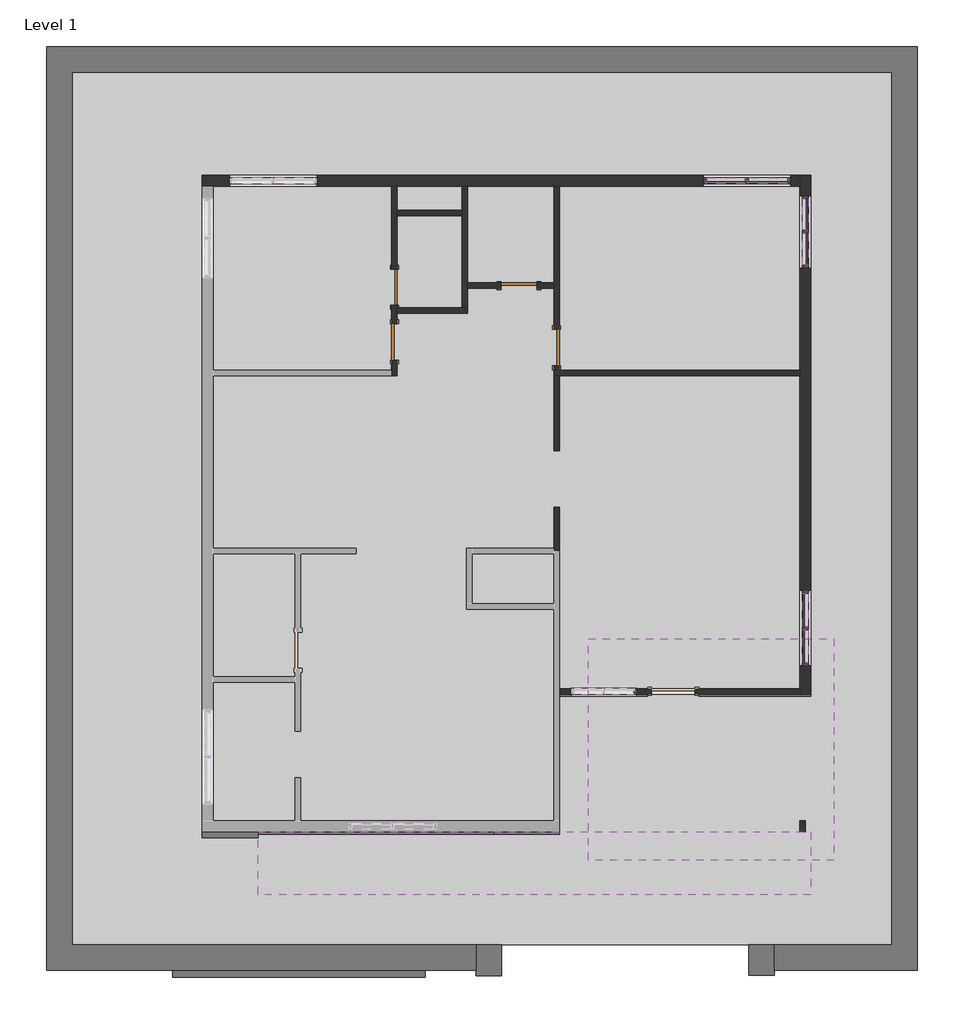
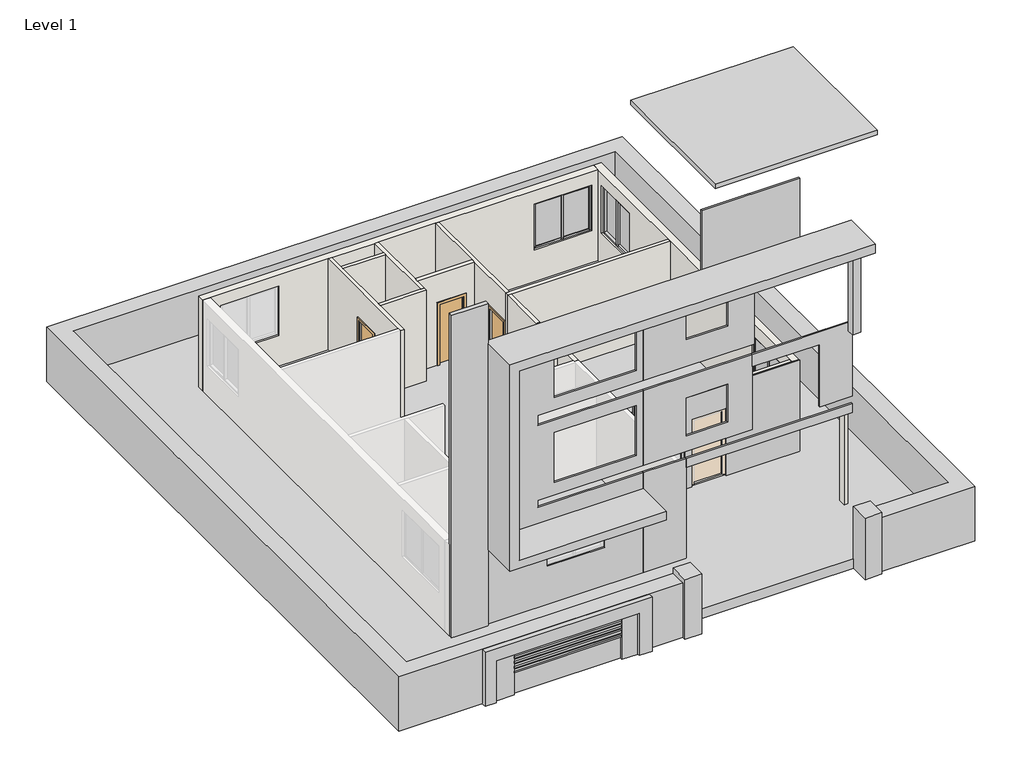
# One storey, part 2 of 2: 22 members, 13 walls, 6 plates, 6 proxies, 4 doors.
"""IFC4 building model written with IfcOpenShell, lengths in millimetres."""

from ifc_helpers import new_model, si_unit, frame, origin, origin_with_axes, place, context, project, spatial, polyline, outline, extrude, faceted_brep, transform, mapped, element, save
from components import generic_models_1_generic_models_1_28fb3979, generic_models_12_generic_models_12_a8744921, generic_models_2_generic_models_2_1119aa77, generic_models_3_generic_models_3_3340ffbe, generic_models_8_generic_models_8_0a5f4393, generic_models_9_generic_models_9_83f75d2b, door_f2b275c1, door_d8f5dbb5, member_5f1d7e17, member_9a58012a, member_18747f1d, member_c33c434a, member_46fa6ebc, member_6998075c, member_c17f1be2, member_2a2664cc, member_2f32d0be, member_c4e92d7b, system_panel_glazed_d989bf7f, system_panel_glazed_5bf0499b, system_panel_glazed_a910ef8c

model = new_model("IFC4")

# Units and contexts
model_context = context("Model", 3, world=origin())
ifc_project = project(units=[si_unit("LENGTHUNIT", "METRE", prefix="MILLI")], contexts=[model_context])

# Site, building, storey
site = spatial("IfcSite", under=ifc_project)
building = spatial("IfcBuilding", under=site)
storey = spatial("IfcBuildingStorey", under=building, Name="Level 1", Elevation=0.0)

# Proxies
placement = place(None, origin())
generic_models_1_generic_models_1_shape = generic_models_1_generic_models_1_28fb3979(model_context)
element("IfcBuildingElementProxy", 1, Name="Generic Models 1 : Generic Models 1", ObjectType="Generic Models 1 : Generic Models 1", at=placement, inside=storey, context=model_context, shape_type="MappedRepresentation", body=[
    mapped(generic_models_1_generic_models_1_shape, transform((0.0, 0.0, 0.0), x_axis=(1.0, 0.0, 0.0), y_axis=(0.0, 1.0, 0.0), z_axis=(0.0, 0.0, 1.0))),
])
generic_models_12_generic_models_12_shape = generic_models_12_generic_models_12_a8744921(model_context)
element("IfcBuildingElementProxy", 2, Name="Generic Models 12 : Generic Models 12", ObjectType="Generic Models 12 : Generic Models 12", at=placement, inside=storey, context=model_context, shape_type="MappedRepresentation", body=[
    mapped(generic_models_12_generic_models_12_shape, transform((0.0, 0.0, 0.0), x_axis=(1.0, 0.0, 0.0), y_axis=(0.0, 1.0, 0.0), z_axis=(0.0, 0.0, 1.0))),
])
generic_models_2_generic_models_2_shape = generic_models_2_generic_models_2_1119aa77(model_context)
element("IfcBuildingElementProxy", 3, Name="Generic Models 2 : Generic Models 2", ObjectType="Generic Models 2 : Generic Models 2", at=placement, inside=storey, context=model_context, shape_type="MappedRepresentation", body=[
    mapped(generic_models_2_generic_models_2_shape, transform((0.0, 0.0, 127.0), x_axis=(1.0, 0.0, 0.0), y_axis=(0.0, 1.0, 0.0), z_axis=(0.0, 0.0, 1.0))),
])
generic_models_3_generic_models_3_shape = generic_models_3_generic_models_3_3340ffbe(model_context)
element("IfcBuildingElementProxy", 4, Name="Generic Models 3 : Generic Models 3", ObjectType="Generic Models 3 : Generic Models 3", at=placement, inside=storey, context=model_context, shape_type="MappedRepresentation", body=[
    mapped(generic_models_3_generic_models_3_shape, transform((0.0, 0.0, 0.0), x_axis=(1.0, 0.0, 0.0), y_axis=(0.0, 1.0, 0.0), z_axis=(0.0, 0.0, 1.0))),
])
generic_models_8_generic_models_8_shape = generic_models_8_generic_models_8_0a5f4393(model_context)
element("IfcBuildingElementProxy", 5, Name="Generic Models 8 : Generic Models 8", ObjectType="Generic Models 8 : Generic Models 8", at=placement, inside=storey, context=model_context, shape_type="MappedRepresentation", body=[
    mapped(generic_models_8_generic_models_8_shape, transform((0.0, 0.0, 0.0), x_axis=(1.0, 0.0, 0.0), y_axis=(0.0, 1.0, 0.0), z_axis=(0.0, 0.0, 1.0))),
])
generic_models_9_generic_models_9_shape = generic_models_9_generic_models_9_83f75d2b(model_context)
element("IfcBuildingElementProxy", 6, Name="Generic Models 9 : Generic Models 9", ObjectType="Generic Models 9 : Generic Models 9", at=placement, inside=storey, context=model_context, shape_type="MappedRepresentation", body=[
    mapped(generic_models_9_generic_models_9_shape, transform((0.0, 0.0, 0.0), x_axis=(1.0, 0.0, 0.0), y_axis=(0.0, 1.0, 0.0), z_axis=(0.0, 0.0, 1.0))),
])

# Doors
door_shape = door_f2b275c1(model_context)
element("IfcDoor", 7, ObjectType="Single-Flush : 30\" x 80\"", at=placement, inside=storey, context=model_context, shape_type="MappedRepresentation", body=[
    mapped(door_shape, transform((-14978.0695233, -3895.4002569, 0.0), x_axis=(0.0, -1.0, 0.0), y_axis=(1.0, 0.0, 0.0), z_axis=(0.0, 0.0, 1.0))),
])
door_2_shape = door_d8f5dbb5(model_context)
element("IfcDoor", 8, ObjectType="Single-Flush : 30\" x 80\"", at=placement, inside=storey, context=model_context, shape_type="MappedRepresentation", body=[
    mapped(door_2_shape, transform((-14978.0695233, -2755.5752569, 0.0), x_axis=(0.0, -1.0, 0.0), y_axis=(1.0, 0.0, 0.0), z_axis=(0.0, 0.0, 1.0))),
])
element("IfcDoor", 9, ObjectType="Single-Flush : 30\" x 80\"", at=placement, inside=storey, context=model_context, shape_type="MappedRepresentation", body=[
    mapped(door_2_shape, transform((-12374.5695233, -2723.8252569, 0.0), x_axis=(1.0, 0.0, 0.0), y_axis=(0.0, 1.0, 0.0), z_axis=(0.0, 0.0, 1.0))),
])
element("IfcDoor", 10, ObjectType="Single-Flush : 30\" x 80\"", at=placement, inside=storey, context=model_context, shape_type="MappedRepresentation", body=[
    mapped(door_2_shape, transform((-11587.1695233, -4019.2252569, 0.0), x_axis=(0.0, -1.0, 0.0), y_axis=(1.0, 0.0, 0.0), z_axis=(0.0, 0.0, 1.0))),
])

# Members
member_shape = member_5f1d7e17(model_context)
element("IfcMember", 11, ObjectType="Rectangular Mullion : 2.5\" x 5\" rectangular", at=placement, inside=storey, context=model_context, shape_type="MappedRepresentation", body=[
    mapped(member_shape, transform((-6386.5195233, -9912.0252569, 2622.4418618), x_axis=(0.0, 0.0, 1.0), y_axis=(1.0, 0.0, 0.0), z_axis=(0.0, 1.0, 0.0))),
])
element("IfcMember", 12, ObjectType="Rectangular Mullion : 2.5\" x 5\" rectangular", at=placement, inside=storey, context=model_context, shape_type="MappedRepresentation", body=[
    mapped(member_shape, transform((-6386.5195233, -9156.3752569, 2622.4418618), x_axis=(0.0, 0.0, 1.0), y_axis=(1.0, 0.0, 0.0), z_axis=(0.0, 1.0, 0.0))),
])
member_2_shape = member_9a58012a(model_context)
element("IfcMember", 13, ObjectType="Rectangular Mullion : 2.5\" x 5\" rectangular", at=placement, inside=storey, context=model_context, shape_type="MappedRepresentation", body=[
    mapped(member_2_shape, transform((-6386.5195233, -9880.2752569, 1032.7455589), x_axis=(0.0, 1.0, 0.0), y_axis=(1.0, 0.0, 0.0), z_axis=(0.0, 0.0, -1.0))),
])
element("IfcMember", 14, ObjectType="Rectangular Mullion : 2.5\" x 5\" rectangular", at=placement, inside=storey, context=model_context, shape_type="MappedRepresentation", body=[
    mapped(member_shape, transform((-6386.5195233, -9848.5252569, 1032.7455589), x_axis=(0.0, 0.0, -1.0), y_axis=(1.0, 0.0, 0.0), z_axis=(0.0, -1.0, 0.0))),
])
element("IfcMember", 15, ObjectType="Rectangular Mullion : 2.5\" x 5\" rectangular", at=placement, inside=storey, context=model_context, shape_type="MappedRepresentation", body=[
    mapped(member_shape, transform((-6386.5195233, -10604.1752569, 1032.7455589), x_axis=(0.0, 0.0, -1.0), y_axis=(1.0, 0.0, 0.0), z_axis=(0.0, -1.0, 0.0))),
])
member_3_shape = member_18747f1d(model_context)
element("IfcMember", 16, ObjectType="Rectangular Mullion : 2.5\" x 5\" rectangular", at=placement, inside=storey, context=model_context, shape_type="MappedRepresentation", body=[
    mapped(member_3_shape, transform((-6386.5195233, -9092.8752569, 1032.7455589), x_axis=(0.0, 1.0, 0.0), y_axis=(1.0, 0.0, 0.0), z_axis=(0.0, 0.0, -1.0))),
])
element("IfcMember", 17, ObjectType="Rectangular Mullion : 2.5\" x 5\" rectangular", at=placement, inside=storey, context=model_context, shape_type="MappedRepresentation", body=[
    mapped(member_3_shape, transform((-6386.5195233, -10667.6752569, 2622.4418618), x_axis=(0.0, -1.0, 0.0), y_axis=(1.0, 0.0, 0.0), z_axis=(0.0, 0.0, 1.0))),
])
member_4_shape = member_c33c434a(model_context)
element("IfcMember", 18, ObjectType="Rectangular Mullion : 2.5\" x 5\" rectangular", at=placement, inside=storey, context=model_context, shape_type="MappedRepresentation", body=[
    mapped(member_4_shape, transform((-6386.5195233, -1568.1252569, 2618.6536186), x_axis=(0.0, 0.0, 1.0), y_axis=(-1.0, 0.0, 0.0), z_axis=(0.0, -1.0, 0.0))),
])
element("IfcMember", 19, ObjectType="Rectangular Mullion : 2.5\" x 5\" rectangular", at=placement, inside=storey, context=model_context, shape_type="MappedRepresentation", body=[
    mapped(member_4_shape, transform((-6386.5195233, -2298.3752569, 2618.6536186), x_axis=(0.0, 0.0, 1.0), y_axis=(-1.0, 0.0, 0.0), z_axis=(0.0, -1.0, 0.0))),
])
member_5_shape = member_46fa6ebc(model_context)
element("IfcMember", 20, ObjectType="Rectangular Mullion : 2.5\" x 5\" rectangular", at=placement, inside=storey, context=model_context, shape_type="MappedRepresentation", body=[
    mapped(member_5_shape, transform((-6386.5195233, -1599.8752569, 1030.540153), x_axis=(0.0, -1.0, 0.0), y_axis=(-1.0, 0.0, 0.0), z_axis=(0.0, 0.0, -1.0))),
])
element("IfcMember", 21, ObjectType="Rectangular Mullion : 2.5\" x 5\" rectangular", at=placement, inside=storey, context=model_context, shape_type="MappedRepresentation", body=[
    mapped(member_4_shape, transform((-6386.5195233, -1631.6252569, 1030.540153), x_axis=(0.0, 0.0, -1.0), y_axis=(-1.0, 0.0, 0.0), z_axis=(0.0, 1.0, 0.0))),
])
element("IfcMember", 22, ObjectType="Rectangular Mullion : 2.5\" x 5\" rectangular", at=placement, inside=storey, context=model_context, shape_type="MappedRepresentation", body=[
    mapped(member_4_shape, transform((-6386.5195233, -901.3752569, 1030.540153), x_axis=(0.0, 0.0, -1.0), y_axis=(-1.0, 0.0, 0.0), z_axis=(0.0, 1.0, 0.0))),
])
member_6_shape = member_6998075c(model_context)
element("IfcMember", 23, ObjectType="Rectangular Mullion : 2.5\" x 5\" rectangular", at=placement, inside=storey, context=model_context, shape_type="MappedRepresentation", body=[
    mapped(member_6_shape, transform((-6386.5195233, -837.8752569, 2618.6536186), x_axis=(0.0, 1.0, 0.0), y_axis=(-1.0, 0.0, 0.0), z_axis=(0.0, 0.0, 1.0))),
])
element("IfcMember", 24, ObjectType="Rectangular Mullion : 2.5\" x 5\" rectangular", at=placement, inside=storey, context=model_context, shape_type="MappedRepresentation", body=[
    mapped(member_6_shape, transform((-6386.5195233, -2361.8752569, 1030.540153), x_axis=(0.0, -1.0, 0.0), y_axis=(-1.0, 0.0, 0.0), z_axis=(0.0, 0.0, -1.0))),
])
member_7_shape = member_c17f1be2(model_context)
element("IfcMember", 25, ObjectType="Rectangular Mullion : 2.5\" x 5\" rectangular", at=placement, inside=storey, context=model_context, shape_type="MappedRepresentation", body=[
    mapped(member_7_shape, transform((-7573.9695233, -533.0752569, 2597.1082833), x_axis=(0.0, 0.0, 1.0), y_axis=(0.0, 1.0, 0.0), z_axis=(-1.0, 0.0, 0.0))),
])
element("IfcMember", 26, ObjectType="Rectangular Mullion : 2.5\" x 5\" rectangular", at=placement, inside=storey, context=model_context, shape_type="MappedRepresentation", body=[
    mapped(member_7_shape, transform((-8456.6195233, -533.0752569, 2597.1082833), x_axis=(0.0, 0.0, 1.0), y_axis=(0.0, 1.0, 0.0), z_axis=(-1.0, 0.0, 0.0))),
])
member_8_shape = member_2a2664cc(model_context)
element("IfcMember", 27, ObjectType="Rectangular Mullion : 2.5\" x 5\" rectangular", at=placement, inside=storey, context=model_context, shape_type="MappedRepresentation", body=[
    mapped(member_8_shape, transform((-7605.7195233, -533.0752569, 1063.3535393), x_axis=(-1.0, 0.0, 0.0), y_axis=(0.0, 1.0, 0.0), z_axis=(0.0, 0.0, -1.0))),
])
element("IfcMember", 28, ObjectType="Rectangular Mullion : 2.5\" x 5\" rectangular", at=placement, inside=storey, context=model_context, shape_type="MappedRepresentation", body=[
    mapped(member_7_shape, transform((-7637.4695233, -533.0752569, 1063.3535393), x_axis=(0.0, 0.0, -1.0), y_axis=(0.0, 1.0, 0.0), z_axis=(1.0, 0.0, 0.0))),
])
element("IfcMember", 29, ObjectType="Rectangular Mullion : 2.5\" x 5\" rectangular", at=placement, inside=storey, context=model_context, shape_type="MappedRepresentation", body=[
    mapped(member_7_shape, transform((-6754.8195233, -533.0752569, 1063.3535393), x_axis=(0.0, 0.0, -1.0), y_axis=(0.0, 1.0, 0.0), z_axis=(1.0, 0.0, 0.0))),
])
member_9_shape = member_2f32d0be(model_context)
element("IfcMember", 30, ObjectType="Rectangular Mullion : 2.5\" x 5\" rectangular", at=placement, inside=storey, context=model_context, shape_type="MappedRepresentation", body=[
    mapped(member_9_shape, transform((-8520.1195233, -533.0752569, 1063.3535393), x_axis=(-1.0, 0.0, 0.0), y_axis=(0.0, 1.0, 0.0), z_axis=(0.0, 0.0, -1.0))),
])
element("IfcMember", 31, ObjectType="Rectangular Mullion : 2.5\" x 5\" rectangular", at=placement, inside=storey, context=model_context, shape_type="MappedRepresentation", body=[
    mapped(member_9_shape, transform((-6691.3195233, -533.0752569, 2597.1082833), x_axis=(1.0, 0.0, 0.0), y_axis=(0.0, 1.0, 0.0), z_axis=(0.0, 0.0, 1.0))),
])
member_10_shape = member_c4e92d7b(model_context)
element("IfcMember", 32, ObjectType="Rectangular Mullion : 2.5\" x 5\" rectangular", at=placement, inside=storey, context=model_context, shape_type="MappedRepresentation", body=[
    mapped(member_10_shape, transform((-9910.7695233, -11201.0752569, 844.8572576), x_axis=(1.0, 0.0, 0.0), y_axis=(0.0, -1.0, 0.0), z_axis=(0.0, 0.0, -1.0))),
])

# Plates
system_panel_glazed_shape = system_panel_glazed_d989bf7f(model_context)
element("IfcPlate", 33, ObjectType="System Panel : Glazed", at=placement, inside=storey, context=model_context, shape_type="MappedRepresentation", body=[
    mapped(system_panel_glazed_shape, transform((-6386.5195233, -10258.1002569, 1096.2455589), x_axis=(0.0, 1.0, 0.0), y_axis=(-1.0, 0.0, 0.0), z_axis=(0.0, 0.0, 1.0))),
])
element("IfcPlate", 34, ObjectType="System Panel : Glazed", at=placement, inside=storey, context=model_context, shape_type="MappedRepresentation", body=[
    mapped(system_panel_glazed_shape, transform((-6386.5195233, -9502.4502569, 1096.2455589), x_axis=(0.0, 1.0, 0.0), y_axis=(-1.0, 0.0, 0.0), z_axis=(0.0, 0.0, 1.0))),
])
system_panel_glazed_2_shape = system_panel_glazed_5bf0499b(model_context)
element("IfcPlate", 35, ObjectType="System Panel : Glazed", at=placement, inside=storey, context=model_context, shape_type="MappedRepresentation", body=[
    mapped(system_panel_glazed_2_shape, transform((-6386.5195233, -1234.7502569, 1094.040153), x_axis=(0.0, -1.0, 0.0), y_axis=(1.0, 0.0, 0.0), z_axis=(0.0, 0.0, 1.0))),
])
element("IfcPlate", 36, ObjectType="System Panel : Glazed", at=placement, inside=storey, context=model_context, shape_type="MappedRepresentation", body=[
    mapped(system_panel_glazed_2_shape, transform((-6386.5195233, -1965.0002569, 1094.040153), x_axis=(0.0, -1.0, 0.0), y_axis=(1.0, 0.0, 0.0), z_axis=(0.0, 0.0, 1.0))),
])
system_panel_glazed_3_shape = system_panel_glazed_a910ef8c(model_context)
element("IfcPlate", 37, ObjectType="System Panel : Glazed", at=placement, inside=storey, context=model_context, shape_type="MappedRepresentation", body=[
    mapped(system_panel_glazed_3_shape, transform((-7164.3945233, -533.0752569, 1126.8535393), x_axis=(-1.0, 0.0, 0.0), y_axis=(0.0, -1.0, 0.0), z_axis=(0.0, 0.0, 1.0))),
])
element("IfcPlate", 38, ObjectType="System Panel : Glazed", at=placement, inside=storey, context=model_context, shape_type="MappedRepresentation", body=[
    mapped(system_panel_glazed_3_shape, transform((-8047.0445233, -533.0752569, 1126.8535393), x_axis=(-1.0, 0.0, 0.0), y_axis=(0.0, -1.0, 0.0), z_axis=(0.0, 0.0, 1.0))),
])

# Walls
element("IfcWall", 39, ObjectType="4.5\"", at=placement, inside=storey, context=model_context, shape_type="Brep", body=[
    faceted_brep([(-15035.2195233, -3136.5752569, 2032.0), (-15035.2195233, -3136.5752569, 0.0), (-15035.2195233, -3514.4002569, 0.0), (-15035.2195233, -3514.4002569, 2032.0), (-15035.2195233, -4276.4002569, 2032.0), (-15035.2195233, -4276.4002569, 0.0), (-15035.2195233, -4495.4752569, 0.0), (-15035.2195233, -4609.7752569, 0.0), (-15035.2195233, -4609.7752569, 3048.0), (-15035.2195233, -4495.4752569, 3048.0), (-15035.2195233, -647.3752569, 3048.0), (-15035.2195233, -647.3752569, 0.0), (-15035.2195233, -2374.5752569, 0.0), (-15035.2195233, -2374.5752569, 2032.0), (-14920.9195233, -3514.4002569, 0.0), (-14920.9195233, -3295.3252569, 0.0), (-14920.9195233, -3181.0252569, 0.0), (-14920.9195233, -3136.5752569, 0.0), (-14920.9195233, -3136.5752569, 2032.0), (-14920.9195233, -2374.5752569, 2032.0), (-14920.9195233, -2374.5752569, 0.0), (-14920.9195233, -1256.9752569, 0.0), (-14920.9195233, -1142.6752569, 0.0), (-14920.9195233, -647.3752569, 0.0), (-14920.9195233, -647.3752569, 3048.0), (-14920.9195233, -1142.6752569, 3048.0), (-14920.9195233, -1256.9752569, 3048.0), (-14920.9195233, -3181.0252569, 3048.0), (-14920.9195233, -3295.3252569, 3048.0), (-14920.9195233, -4609.7752569, 3048.0), (-14920.9195233, -4609.7752569, 0.0), (-14920.9195233, -4276.4002569, 0.0), (-14920.9195233, -4276.4002569, 2032.0), (-14920.9195233, -3514.4002569, 2032.0)], [[[0, 1, 2, 3, 4, 5, 6, 7, 8, 9, 10, 11, 12, 13]], [[14, 15, 16, 17, 18, 19, 20, 21, 22, 23, 24, 25, 26, 27, 28, 29, 30, 31, 32, 33]], [[7, 6, 5, 31, 30]], [[12, 11, 23, 22, 21, 20]], [[2, 1, 17, 16, 15, 14]], [[10, 9, 8, 29, 28, 27, 26, 25, 24]], [[11, 10, 24, 23]], [[8, 7, 30, 29]], [[32, 31, 5, 4]], [[33, 32, 4, 3]], [[14, 33, 3, 2]], [[18, 17, 1, 0]], [[19, 18, 0, 13]], [[20, 19, 13, 12]]]),
])
element("IfcWall", 40, ObjectType="4.5\"", at=placement, inside=storey, context=model_context, shape_type="Brep", body=[
    faceted_brep([(-13568.3695233, -647.3752569, 0.0), (-13568.3695233, -1142.6752569, 0.0), (-13568.3695233, -1256.9752569, 0.0), (-13568.3695233, -3181.0252569, 0.0), (-13568.3695233, -3181.0252569, 3048.0), (-13568.3695233, -1256.9752569, 3048.0), (-13568.3695233, -1142.6752569, 3048.0), (-13568.3695233, -647.3752569, 3048.0), (-13454.0695233, -647.3752569, 0.0), (-13454.0695233, -647.3752569, 3048.0), (-13454.0695233, -2666.6752569, 3048.0), (-13454.0695233, -2780.9752569, 3048.0), (-13454.0695233, -3181.0252569, 3048.0), (-13454.0695233, -3181.0252569, 0.0), (-13454.0695233, -2780.9752569, 0.0), (-13454.0695233, -2666.6752569, 0.0)], [[[0, 1, 2, 3, 4, 5, 6, 7]], [[8, 9, 10, 11, 12, 13, 14, 15]], [[3, 2, 1, 0, 8, 15, 14, 13]], [[7, 6, 5, 4, 12, 11, 10, 9]], [[0, 7, 9, 8]], [[4, 3, 13, 12]]]),
])
element("IfcWall", 41, ObjectType="4.5\"", at=placement, inside=storey, context=model_context, shape_type="SweptSolid", body=[
    extrude(outline(polyline([(-14920.9195233, -1142.6752569), (-13568.3695233, -1142.6752569), (-13568.3695233, -1256.9752569), (-14920.9195233, -1256.9752569), (-14920.9195233, -1142.6752569)])), origin_with_axes(), (0.0, 0.0, 1.0), 3048.0),
])
element("IfcWall", 42, ObjectType="4.5\"", at=placement, inside=storey, context=model_context, shape_type="Brep", body=[
    faceted_brep([(-14920.9195233, -3295.3252569, 0.0), (-13454.0695233, -3295.3252569, 0.0), (-13454.0695233, -3295.3252569, 3048.0), (-14920.9195233, -3295.3252569, 3048.0), (-14920.9195233, -3181.0252569, 0.0), (-14920.9195233, -3181.0252569, 3048.0), (-13568.3695233, -3181.0252569, 3048.0), (-13454.0695233, -3181.0252569, 3048.0), (-13454.0695233, -3181.0252569, 0.0), (-13568.3695233, -3181.0252569, 0.0)], [[[0, 1, 2, 3]], [[4, 5, 6, 7, 8, 9]], [[1, 0, 4, 9, 8]], [[3, 2, 7, 6, 5]], [[0, 3, 5, 4]], [[2, 1, 8, 7]]]),
])
element("IfcWall", 43, ObjectType="4.5\"", at=placement, inside=storey, context=model_context, shape_type="Brep", body=[
    faceted_brep([(-11644.3195233, -4400.2252569, 2032.0), (-11644.3195233, -4400.2252569, 0.0), (-11644.3195233, -4495.4752569, 0.0), (-11644.3195233, -4495.4752569, 3048.0), (-11644.3195233, -2780.9752569, 3048.0), (-11644.3195233, -2666.6752569, 3048.0), (-11644.3195233, -647.3752569, 3048.0), (-11644.3195233, -647.3752569, 0.0), (-11644.3195233, -2666.6752569, 0.0), (-11644.3195233, -2780.9752569, 0.0), (-11644.3195233, -3638.2252569, 0.0), (-11644.3195233, -3638.2252569, 2032.0), (-11530.0195233, -4495.4752569, 0.0), (-11530.0195233, -4400.2252569, 0.0), (-11530.0195233, -4400.2252569, 2032.0), (-11530.0195233, -3638.2252569, 2032.0), (-11530.0195233, -3638.2252569, 0.0), (-11530.0195233, -647.3752569, 0.0), (-11530.0195233, -647.3752569, 3048.0), (-11530.0195233, -4495.4752569, 3048.0)], [[[0, 1, 2, 3, 4, 5, 6, 7, 8, 9, 10, 11]], [[12, 13, 14, 15, 16, 17, 18, 19]], [[2, 1, 13, 12]], [[10, 9, 8, 7, 17, 16]], [[6, 5, 4, 3, 19, 18]], [[7, 6, 18, 17]], [[3, 2, 12, 19]], [[14, 13, 1, 0]], [[15, 14, 0, 11]], [[16, 15, 11, 10]]]),
])
element("IfcWall", 44, ObjectType="4.5\"", at=placement, inside=storey, context=model_context, shape_type="SweptSolid", body=[
    extrude(outline(polyline([(2032.0, -11993.5695233), (0.0, -11993.5695233), (0.0, -11644.3195233), (3048.0, -11644.3195233), (3048.0, -13454.0695233), (0.0, -13454.0695233), (0.0, -12755.5695233), (2032.0, -12755.5695233), (2032.0, -11993.5695233)])), frame((0.0, -2780.9752569, 0.0), z_axis=(0.0, 1.0, 0.0), x_axis=(0.0, 0.0, 1.0)), (0.0, 0.0, 1.0), 114.3),
])
element("IfcWall", 45, ObjectType="4.5\"", at=placement, inside=storey, context=model_context, shape_type="Brep", body=[
    faceted_brep([(-11644.3195233, -4609.7752569, 0.0), (-11530.0195233, -4609.7752569, 0.0), (-6500.8195233, -4609.7752569, 0.0), (-6500.8195233, -4609.7752569, 3048.0), (-11530.0195233, -4609.7752569, 3048.0), (-11644.3195233, -4609.7752569, 3048.0), (-11644.3195233, -4495.4752569, 0.0), (-11644.3195233, -4495.4752569, 3048.0), (-11530.0195233, -4495.4752569, 3048.0), (-6500.8195233, -4495.4752569, 3048.0), (-6500.8195233, -4495.4752569, 0.0), (-11530.0195233, -4495.4752569, 0.0)], [[[0, 1, 2, 3, 4, 5]], [[6, 7, 8, 9, 10, 11]], [[2, 1, 0, 6, 11, 10]], [[5, 4, 3, 9, 8, 7]], [[3, 2, 10, 9]], [[0, 5, 7, 6]]]),
])
element("IfcWall", 46, ObjectType="4.5\"", at=placement, inside=storey, context=model_context, shape_type="SweptSolid", body=[
    extrude(outline(polyline([(-11644.3195233, -6178.2252569), (-11644.3195233, -4609.7752569), (-11530.0195233, -4609.7752569), (-11530.0195233, -6178.2252569), (-11644.3195233, -6178.2252569)])), origin_with_axes(), (0.0, 0.0, 1.0), 3048.0),
])
element("IfcWall", 47, ObjectType="4.5\"", at=placement, inside=storey, context=model_context, shape_type="SweptSolid", body=[
    extrude(outline(polyline([(0.0, -11530.0195233), (0.0, -6500.8195233), (3048.0, -6500.8195233), (3048.0, -11530.0195233), (0.0, -11530.0195233)]), holes=[polyline([(50.8, -8691.5695233), (50.8, -9605.9695233), (2184.4, -9605.9695233), (2184.4, -8691.5695233), (50.8, -8691.5695233)]), polyline([(844.8572576, -11282.3695233), (2316.9077492, -11282.3695233), (2316.9077492, -9910.7695233), (844.8572576, -9910.7695233), (844.8572576, -11282.3695233)])]), frame((0.0, -11258.2252569, 0.0), z_axis=(0.0, 1.0, 0.0), x_axis=(0.0, 0.0, 1.0)), (0.0, 0.0, 1.0), 114.3),
])
element("IfcWall", 48, ObjectType="4.5\"", at=placement, inside=storey, context=model_context, shape_type="Brep", body=[
    faceted_brep([(-11644.3195233, -7352.9752569, 0.0), (-11644.3195233, -8210.2252569, 0.0), (-11644.3195233, -8267.3752569, 0.0), (-11644.3195233, -8267.3752569, 3048.0), (-11644.3195233, -8210.2252569, 3048.0), (-11644.3195233, -7352.9752569, 3048.0), (-11530.0195233, -7352.9752569, 0.0), (-11530.0195233, -7352.9752569, 3048.0), (-11530.0195233, -8267.3752569, 3048.0), (-11530.0195233, -8267.3752569, 0.0)], [[[0, 1, 2, 3, 4, 5]], [[6, 7, 8, 9]], [[2, 1, 0, 6, 9]], [[3, 2, 9, 8]], [[5, 4, 3, 8, 7]], [[0, 5, 7, 6]]]),
])
element("IfcWall", 49, ObjectType="9\"", at=placement, inside=storey, context=model_context, shape_type="Brep", body=[
    faceted_brep([(-6500.8195233, -418.7752569, 0.0), (-18997.6195233, -418.7752569, 0.0), (-18997.6195233, -418.7752569, 3048.0), (-6500.8195233, -418.7752569, 3048.0), (-6691.3195233, -418.7752569, 1063.3535393), (-6691.3195233, -418.7752569, 2597.1082833), (-8520.1195233, -418.7752569, 2597.1082833), (-8520.1195233, -418.7752569, 1063.3535393), (-18426.1195233, -418.7752569, 2671.7497986), (-18426.1195233, -418.7752569, 1031.9306853), (-16597.3195233, -418.7752569, 1031.9306853), (-16597.3195233, -418.7752569, 2671.7497986), (-18997.6195233, -647.3752569, 0.0), (-18769.0195233, -647.3752569, 0.0), (-15035.2195233, -647.3752569, 0.0), (-14920.9195233, -647.3752569, 0.0), (-13568.3695233, -647.3752569, 0.0), (-13454.0695233, -647.3752569, 0.0), (-11644.3195233, -647.3752569, 0.0), (-11530.0195233, -647.3752569, 0.0), (-6500.8195233, -647.3752569, 0.0), (-6500.8195233, -647.3752569, 3048.0), (-11530.0195233, -647.3752569, 3048.0), (-11644.3195233, -647.3752569, 3048.0), (-13454.0695233, -647.3752569, 3048.0), (-13568.3695233, -647.3752569, 3048.0), (-14920.9195233, -647.3752569, 3048.0), (-15035.2195233, -647.3752569, 3048.0), (-18769.0195233, -647.3752569, 3048.0), (-18997.6195233, -647.3752569, 3048.0), (-6691.3195233, -647.3752569, 2597.1082833), (-6691.3195233, -647.3752569, 1063.3535393), (-8520.1195233, -647.3752569, 1063.3535393), (-8520.1195233, -647.3752569, 2597.1082833), (-18426.1195233, -647.3752569, 1031.9306853), (-18426.1195233, -647.3752569, 2671.7497986), (-16597.3195233, -647.3752569, 2671.7497986), (-16597.3195233, -647.3752569, 1031.9306853)], [[[0, 1, 2, 3], [4, 5, 6, 7], [8, 9, 10, 11]], [[12, 13, 14, 15, 16, 17, 18, 19, 20, 21, 22, 23, 24, 25, 26, 27, 28, 29], [30, 31, 32, 33], [34, 35, 36, 37]], [[1, 0, 20, 19, 18, 17, 16, 15, 14, 13, 12]], [[3, 2, 29, 28, 27, 26, 25, 24, 23, 22, 21]], [[0, 3, 21, 20]], [[2, 1, 12, 29]], [[4, 31, 30, 5]], [[5, 30, 33, 6]], [[6, 33, 32, 7]], [[31, 4, 7, 32]], [[34, 9, 8, 35]], [[35, 8, 11, 36]], [[10, 37, 36, 11]], [[9, 34, 37, 10]]]),
])
element("IfcWall", 50, ObjectType="9\"", at=placement, inside=storey, context=model_context, shape_type="SweptSolid", body=[
    extrude(outline(polyline([(-6386.5195233, -14134.7752569), (-6500.8195233, -14134.7752569), (-6500.8195233, -13906.1752569), (-6386.5195233, -13906.1752569), (-6386.5195233, -14134.7752569)])), origin_with_axes(), (0.0, 0.0, 1.0), 3048.0),
])
element("IfcWall", 51, ObjectType="9\"", at=placement, inside=storey, context=model_context, shape_type="Brep", body=[
    faceted_brep([(-6272.2195233, -11258.2252569, 0.0), (-6272.2195233, -418.7752569, 0.0), (-6272.2195233, -418.7752569, 3048.0), (-6272.2195233, -11258.2252569, 3048.0), (-6272.2195233, -837.8752569, 2618.6536186), (-6272.2195233, -837.8752569, 1030.540153), (-6272.2195233, -2361.8752569, 1030.540153), (-6272.2195233, -2361.8752569, 2618.6536186), (-6272.2195233, -10667.6752569, 1032.7455589), (-6272.2195233, -10667.6752569, 2622.4418618), (-6272.2195233, -9092.8752569, 2622.4418618), (-6272.2195233, -9092.8752569, 1032.7455589), (-6500.8195233, -418.7752569, 0.0), (-6500.8195233, -647.3752569, 0.0), (-6500.8195233, -4495.4752569, 0.0), (-6500.8195233, -4609.7752569, 0.0), (-6500.8195233, -11143.9252569, 0.0), (-6500.8195233, -11258.2252569, 0.0), (-6500.8195233, -11258.2252569, 3048.0), (-6500.8195233, -11143.9252569, 3048.0), (-6500.8195233, -4609.7752569, 3048.0), (-6500.8195233, -4495.4752569, 3048.0), (-6500.8195233, -647.3752569, 3048.0), (-6500.8195233, -418.7752569, 3048.0), (-6500.8195233, -837.8752569, 1030.540153), (-6500.8195233, -837.8752569, 2618.6536186), (-6500.8195233, -2361.8752569, 2618.6536186), (-6500.8195233, -2361.8752569, 1030.540153), (-6500.8195233, -10667.6752569, 2622.4418618), (-6500.8195233, -10667.6752569, 1032.7455589), (-6500.8195233, -9092.8752569, 1032.7455589), (-6500.8195233, -9092.8752569, 2622.4418618)], [[[0, 1, 2, 3], [4, 5, 6, 7], [8, 9, 10, 11]], [[12, 13, 14, 15, 16, 17, 18, 19, 20, 21, 22, 23], [24, 25, 26, 27], [28, 29, 30, 31]], [[1, 0, 17, 16, 15, 14, 13, 12]], [[3, 2, 23, 22, 21, 20, 19, 18]], [[0, 3, 18, 17]], [[2, 1, 12, 23]], [[24, 5, 4, 25]], [[25, 4, 7, 26]], [[6, 27, 26, 7]], [[5, 24, 27, 6]], [[8, 29, 28, 9]], [[9, 28, 31, 10]], [[10, 31, 30, 11]], [[29, 8, 11, 30]]]),
])

save(model, "model.ifc")

# Revit data of these elements
# Type "Single-Flush : 30\" x 80\""
#   Type Mark = "5"
#   Construction Type Id = "MDOOR"
#   Assembly Code = "C1020"
#   Analytic Construction = "Metal"
#   Thickness = 0' - 2"
#   Heat Transfer Coefficient (U) = 0.651978 BTU/(h·ft²·°F)
#   Height = 6' - 8"
#   Trim Projection Ext = 0' - 1"
#   Trim Projection Int = 0' - 1"
#   Trim Width = 0' - 3"
#   Width = 2' - 6"
#   Define Thermal Properties by = 1
#   Define Thermal Properties by = 1
#   Door Material = Door - Panel
#   Frame Material = Door - Frame
#   Visual Light Transmittance = 0
#   Solar Heat Gain Coefficient = 0
#   Function = (empty or 0)
#   Wall Closure = (empty or 0)
# Type "Rectangular Mullion : 2.5\" x 5\" rectangular"
#   built-in parameter 1007304 = 0.416667 (stored number, unit not read)
#   built-in parameter 1007301 = 0.104167 (stored number, unit not read)
#   built-in parameter 1007300 = 0.104167 (stored number, unit not read)
# Type "System Panel : Glazed"
#   Construction Type Id = "GSP4R"
#   Analytic Construction = "1/8 in Pilkington single glazing"
#   Visual Light Transmittance = 0.9
#   Solar Heat Gain Coefficient = 0.86
#   Heat Transfer Coefficient (U) = 1.18115 BTU/(h·ft²·°F)
#   Define Thermal Properties by = 1
# Type "4.5\""
#   Assembly Code = "B2010"
#   Layers, outside or top first: 0' - 4 1/2" no material (function 1)
# Type "9\""
#   Assembly Code = "B2010"
#   Layers, outside or top first: 0' - 9" no material (function 1)
# Element 1 (IfcBuildingElementProxy, "Generic Models 1 : Generic Models 1")
#   Phase Created = New Construction
# Element 2 (IfcBuildingElementProxy, "Generic Models 12 : Generic Models 12")
#   Phase Created = New Construction
# Element 3 (IfcBuildingElementProxy, "Generic Models 2 : Generic Models 2")
#   Phase Created = New Construction
# Element 4 (IfcBuildingElementProxy, "Generic Models 3 : Generic Models 3")
#   Phase Created = New Construction
# Element 5 (IfcBuildingElementProxy, "Generic Models 8 : Generic Models 8")
#   Phase Created = New Construction
# Element 6 (IfcBuildingElementProxy, "Generic Models 9 : Generic Models 9")
#   Phase Created = New Construction
# Elements 7, 8, 9, 10 (IfcDoor, "Single-Flush : 30\" x 80\"")
#   Phase Created = New Construction
#   Materials on its faces: "Door - Frame", "Door - Panel"
# Elements 11, 12, 13, 14, 15, 16, 17, 18, 19, 20, 21, 22, 23, 24, 25, 26, 27, 28, 29, 30, 31, 32 (IfcMember, "Rectangular Mullion : 2.5\" x 5\" rectangular")
#   Phase Created = New Construction
#   Materials on its faces: "Aluminum"
# Elements 33, 34, 35, 36, 37, 38 (IfcPlate, "System Panel : Glazed")
#   Phase Created = New Construction
#   Materials on its faces: "Glass"
# Elements 39, 40, 41, 42, 43, 44, 45, 46, 47, 48 (IfcWall, "4.5\"")
#   Top Offset = 0' - 0"
#   Base Offset = 0' - 0"
#   Unconnected Height = 10' - 0"
#   wall height = 10' - 0"
#   Phase Created = New Construction
#   Base Constraint = Level 1
#   Materials on its faces: "Default Wall"
# Elements 49, 50, 51 (IfcWall, "9\"")
#   Top Offset = 0' - 0"
#   Base Offset = 0' - 0"
#   Unconnected Height = 10' - 0"
#   wall height = 10' - 0"
#   Phase Created = New Construction
#   Base Constraint = Level 1
#   Materials on its faces: "Default Wall"
# Materials
#   "Door - Panel": class "Wood", colour RGB 210 159 95, transparency 0, Cost = 0
#   "Door - Frame": colour RGB 118 70 51, transparency 0, Cost = 0
#   "Aluminum": class "Metal", colour RGB 247 247 247, transparency 0, Description = "Aluminum 6061", Cost = 0
#   "Glass": class "Glass", colour RGB 0 128 192, transparency 0.75, Description = "Soda Lime Glass", Cost = 0
#   "Default Wall": colour RGB 128 128 128, transparency 0, Cost = 0
